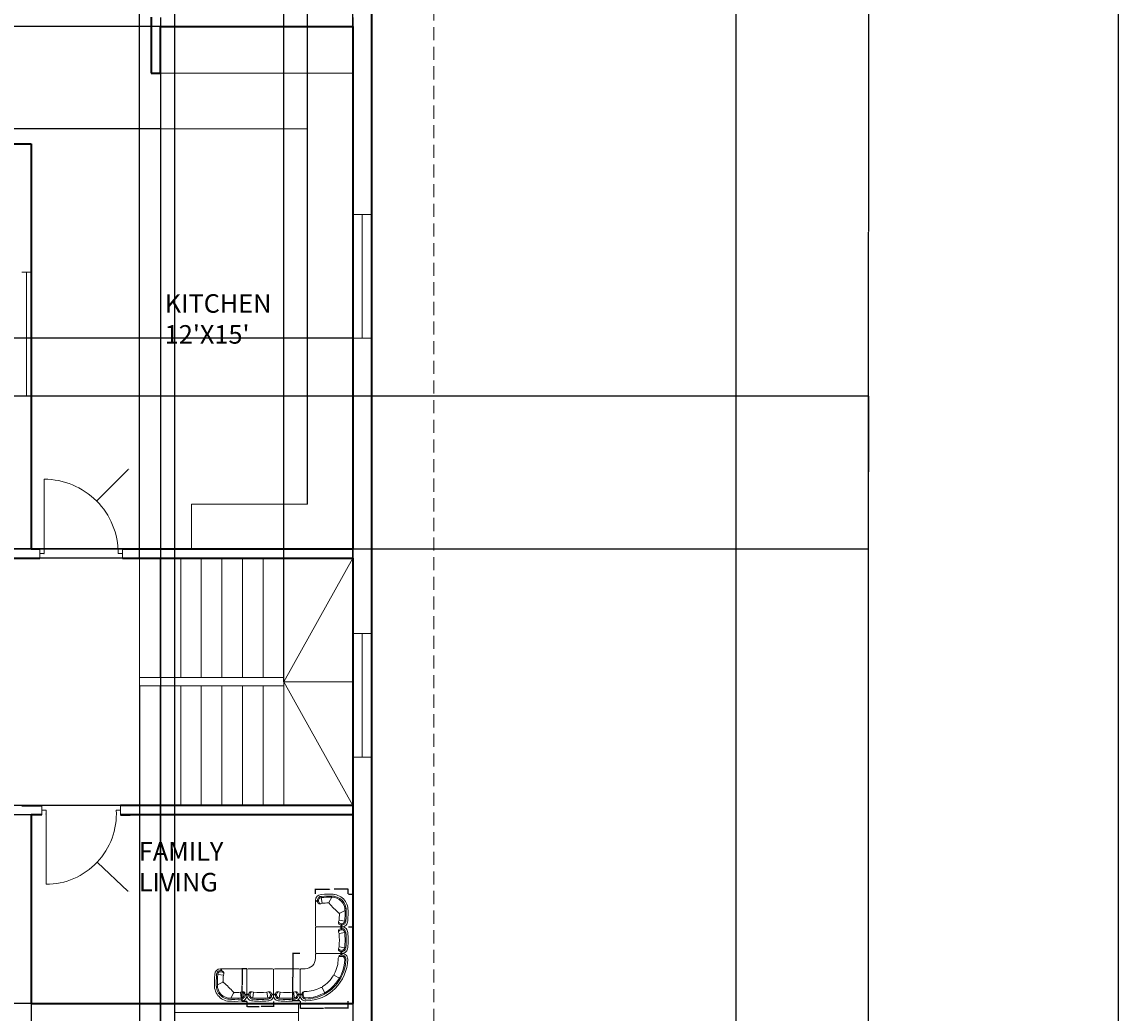
# Model space of a CAD drawing. Units: inches. Extents: x 1770 to 2988, y 1161 to 3221.
# Tile 21 of 44: x 2456 to 2988, y 1614 to 2095. Entities that reach past the tile are written whole.
import ezdxf

# ---------------------------------------------------------------- set-up
doc = ezdxf.new("R2010")
doc.units = ezdxf.units.IN
doc.linetypes.add('DASHED2', pattern=[9.525, 6.35, -3.175])
for name, color, linetype, lineweight in [('A-ANNO-DIMS', 2, 'Continuous', 18), ('A-ANNO-TTLB', 7, 'Continuous', 25), ('A-AREA-IDEN', 7, 'Continuous', 18), ('A-DOOR', 4, 'Continuous', 18), ('A-FLOR-CASE', 8, 'Continuous', 18), ('A-FLOR-STRS', 7, 'Continuous', 18), ('A-FURN', 8, 'Continuous', 13), ('A-GLAZ', 4, 'Continuous', 18), ('A-ROOF-OVHD', 7, 'DASHED2', 18), ('A-WALL', 7, 'Continuous', 35), ('C-PROP', 7, 'Continuous', 25)]:
    doc.layers.add(name, color=color, linetype=linetype, lineweight=lineweight)
doc.styles.get("Standard").update_dxf_attribs({"font": 'arial.ttf'})
doc.dimstyles.get("Standard").update_dxf_attribs({"dimtxt": 0.18, "dimasz": 0.18, "dimexe": 0.18, "dimexo": 0.0625, "dimgap": 0.09, "dimtad": 0, "dimtih": 1, "dimtoh": 1, "dimdec": 4, "dimzin": 0, "dimdsep": 46, "dimtxsty": 'Standard', "dimcen": 0.09, "dimadec": 0, "dimazin": 0, "dimtfac": 1, "dimtdec": 4, "dimtofl": 0, "dimtmove": 0, "dimatfit": 3, "dimfxl": 1, "dimtolj": 1, "dimtzin": 0, "dimarcsym": 0})

# ---------------------------------------------------------------- blocks, each defined once
blk = doc.blocks.new('A$C707258B2')
at = {"color": 0}
for p, q in [((0.404, 0.342), (1.074, 0.342)), ((0.404, 0.292), (0.454, 0.292)), ((1.104, 0.312), (1.104, 0.212)), ((0.404, 0.262), (0.454, 0.262)), ((0.6, -0.238), (0.47, -0.313)), ((1.479, -0.063), (1.379, -0.063)), ((1.509, -0.763), (1.509, -0.093)), ((0.929, -0.567), (0.854, -0.697)), ((1.429, -0.763), (1.429, -0.713)), ((1.459, -0.763), (1.459, -0.712))]:
    blk.add_line(p, q, dxfattribs=at)
for centre, radius, start, end in [((0.404, 0.192), 0.15, 90, 181.1754), ((0.404, 0.192), 0.1, 90, 181.1754), ((0.378, 0.317), 0.0362, 316.3972, 43.6028), ((0.368, 0.317), 0.0662, 337.8298, 22.1702), ((0.455, 0.256), 0.0357, 345.4262, 90.5555), ((1.074, 0.312), 0.03, 360, 90), ((1.379, 0.212), 1.125, 181.1754, 268.8246), ((1.379, 0.212), 1.075, 181.1754, 208.6357), ((0.404, 0.192), 0.07, 90, 181.1754), ((1.379, 0.212), 1.045, 181.1754, 268.8246), ((0.454, 0.212), 0.05, 360, 90), ((1.379, 0.212), 0.875, 180, 208.4082), ((1.379, 0.212), 0.275, 180, 270), ((0.587, -0.216), 0.025, 300, 28.4082), ((0.612, -0.259), 0.025, 31.5918, 120), ((1.379, 0.212), 0.875, 211.5918, 238.4082), ((1.479, -0.093), 0.03, 360, 90), ((0.457, -0.291), 0.025, 208.6357, 300), ((0.482, -0.334), 0.025, 120, 211.3643), ((1.379, 0.212), 1.075, 211.3643, 238.6357), ((0.907, -0.555), 0.025, 330, 58.4082), ((0.951, -0.58), 0.025, 61.5918, 150), ((1.379, 0.212), 0.875, 241.5918, 270), ((0.832, -0.685), 0.025, 238.6357, 330), ((0.876, -0.71), 0.025, 150, 241.3643), ((1.379, 0.212), 1.075, 241.3643, 268.8246), ((1.359, -0.763), 0.15, 268.8246, 360), ((1.359, -0.763), 0.1, 268.8246, 360), ((1.359, -0.763), 0.07, 268.8246, 360), ((1.379, -0.713), 0.05, 360, 90), ((1.425, -0.709), 0.0336, 354.6301, 109.3883), ((1.484, -0.799), 0.0662, 67.8298, 112.1702), ((1.484, -0.789), 0.0362, 46.3972, 133.6028)]:
    blk.add_arc(centre, radius, start, end, dxfattribs=at)
blk = doc.blocks.new('part 01')
at = {"color": 0}
for p, q in [((-670, 700), (0, 700)), ((30, 30), (30, 670)), ((-591, 527), (-740, 550)), ((-591, 527), (-579, 561)), ((-591, 173), (-740, 150)), ((-670, 0), (0, 0)), ((-591, 173), (-579, 139))]:
    blk.add_line(p, q, dxfattribs=at)
for centre, radius, start, end in [((-670, 550), 150, 90, 181.1754), ((-670, 550), 100, 90, 181.1754), ((-670, 550), 70, 90, 181.1754), ((-660, 518), 133, 56.0897, 95.6132), ((-696, 675), 36.2, 316.3972, 43.6028), ((-660, 518), 103, 42.0066, 95.6132), ((-706, 675), 66.2, 337.8298, 22.1702), ((-600, 607), 25, 332.9608, 56.0897), ((-625, 620), 53.2, 321.0017, 332.9608), ((-602, 570), 25, 340, 42.0066), ((0, 670), 30, 0, 90), ((1178, 350), 2008, 174.2835, 185.7165), ((1178, 350), 1958, 174.2835, 185.7165), ((1178, 350), 1928, 174.2835, 185.7165), ((1178, 350), 1778, 174.2835, 185.7165), ((-670, 150), 150, 178.8246, 270), ((-670, 150), 100, 178.8246, 270), ((-670, 150), 70, 178.8246, 270), ((-660, 182), 133, 264.3868, 303.9103), ((-660, 182), 103, 264.3868, 317.9934), ((-696, 25), 36.2, 316.3972, 43.6028), ((-706, 25), 66.2, 337.8298, 22.1702), ((-600, 93), 25, 303.9103, 27.0392), ((-602, 130), 25, 317.9934, 20), ((-625, 80), 53.2, 27.0392, 38.9983), ((0, 30), 30, 270, 0)]:
    blk.add_arc(centre, radius, start, end, dxfattribs=at)
blk = doc.blocks.new('part02')
at = {"color": 0}
for p, q in [((0, -670), (0, 0)), ((30, 30), (700, 30)), ((621, -143), (609, -109)), ((621, -143), (770, -120)), ((640, -326), (778, -399)), ((173, -591), (139, -579)), ((173, -591), (150, -740)), ((356, -610), (429, -748))]:
    blk.add_line(p, q, dxfattribs=at)
for centre, radius, start, end in [((30, 0), 30, 90, 180), ((726, 5), 56.2, 153.6122, 206.6666), ((726, 5), 36.2, 136.3972, 223.6028), ((700, -120), 150, 0, 90), ((630, -63), 25, 123.9103, 207.0392), ((655, -50), 53.2, 207.0392, 218.9983), ((632, -100), 25, 137.9934, 200), ((690, -152), 103, 84.3868, 137.9934), ((689, -151), 132, 85.4378, 123.9887), ((-1148, -320), 1778, 0.3836, 5.7165), ((700, -121), 101, 357.5006, 89.858), ((700, -120), 70, 0, 90), ((-1228, -320), 2008, 357.7349, 5.7032), ((-1148, -320), 1958, 355.8657, 5.7165), ((-1148, -320), 2008, 355.818, 5.7165), ((93, -600), 25, 62.9608, 146.0897), ((80, -625), 53.2, 51.0017, 62.9608), ((130, -602), 25, 70, 132.0066), ((2220, -2190), 2454, 130.6961, 139.3039), ((439, -409), 419, 268.2181, 1.7819), ((439, -409), 369, 268.2181, 1.7819), ((439, -409), 339, 268.2181, 1.7819), ((632, -344), 20, 62, 130.6961), ((650, -308), 20, 180.3836, 242), ((25, -696), 56.2, 63.3334, 116.3878), ((25, -696), 36.2, 46.3972, 133.6028), ((150, -670), 150, 180, 271.1754), ((182, -660), 133, 146.0897, 185.6132), ((150, -670), 100, 180, 271.1754), ((182, -660), 103, 132.0066, 185.6132), ((150, -670), 70, 180, 270), ((350, 1258), 2008, 264.2968, 272.2651), ((350, 1178), 2008, 264.2835, 274.182), ((350, 1178), 1958, 264.2835, 274.1343), ((350, 1178), 1778, 264.2835, 269.6164), ((338, -620), 20, 28, 89.6164), ((374, -602), 20, 139.3039, 208)]:
    blk.add_arc(centre, radius, start, end, dxfattribs=at)
blk = doc.blocks.new('WIN-60-EXT')
for p, q in [((0, 9), (0, 0)), ((60, 4.5), (60, 9)), ((60, 9), (60, 0)), ((0, 0), (0, 4.5)), ((0, 4.5), (60, 4.5))]:
    blk.add_line(p, q)
blk = doc.blocks.new('WIN-60-COURTYARD')
for p, q in [((0, 4.5), (0, 0)), ((0, 0), (0, 2.25)), ((0, 2.25), (60, 2.25)), ((60, 2.25), (60, 4.5)), ((60, 4.5), (60, 0))]:
    blk.add_line(p, q)
blk = doc.blocks.new('*D44')
at = {"layer": 'A-ANNO-DIMS', "color": 0, "lineweight": -2, "transparency": 16777216}
for p, q in [((2565.27, 1635.99), (2562.77, 1635.99)), ((2562.95, 1635.81), (2562.95, 1628.23)), ((2562.95, 1620.29), (2562.95, 1627.87)), ((2565.27, 1620.11), (2562.77, 1620.11))]:
    blk.add_line(p, q, dxfattribs=at)
at = {"layer": 'A-ANNO-DIMS', "color": 0, "transparency": 16777216}
for points in [[(2562.92, 1635.81), (2562.98, 1635.81), (2562.95, 1635.99)], [(2562.92, 1620.29), (2562.98, 1620.29), (2562.95, 1620.11)]]:
    blk.add_solid(points, dxfattribs=at)
at = {"layer": 'Defpoints', "color": 0, "transparency": 16777216}
for p in [(2562.95, 1635.99), (2565.33, 1635.99), (2565.33, 1620.11)]:
    blk.add_point(p, dxfattribs=at)
at = {"layer": 'A-ANNO-DIMS', "color": 0, "transparency": 16777216, "insert": (2562.95, 1628.05), "char_height": 0.18, "attachment_point": 5}
blk.add_mtext('\\A1;SEAT 16 TYP.', dxfattribs=at)
blk = doc.blocks.new('*D45')
at = {"layer": 'A-ANNO-DIMS', "color": 0, "lineweight": -2, "transparency": 16777216}
for p, q in [((2565.33, 1620.05), (2565.33, 1617.55)), ((2565.51, 1617.73), (2571.25, 1617.73)), ((2578.04, 1617.73), (2572.29, 1617.73)), ((2578.22, 1620.05), (2578.22, 1617.55))]:
    blk.add_line(p, q, dxfattribs=at)
at = {"layer": 'A-ANNO-DIMS', "color": 0, "transparency": 16777216}
for points in [[(2565.51, 1617.76), (2565.51, 1617.7), (2565.33, 1617.73)], [(2578.04, 1617.76), (2578.04, 1617.7), (2578.22, 1617.73)]]:
    blk.add_solid(points, dxfattribs=at)
at = {"layer": 'Defpoints', "color": 0, "transparency": 16777216}
for p in [(2565.33, 1620.11), (2565.33, 1617.73), (2578.22, 1620.11)]:
    blk.add_point(p, dxfattribs=at)
at = {"layer": 'A-ANNO-DIMS', "color": 0, "transparency": 16777216, "insert": (2571.77, 1617.73), "char_height": 0.18, "attachment_point": 5}
blk.add_mtext('\\A1;13 TYP.', dxfattribs=at)
blk = doc.blocks.new('*D46')
at = {"layer": 'A-ANNO-DIMS', "color": 0, "lineweight": -2, "transparency": 16777216}
for p, q in [((2598.55, 1672.27), (2598.55, 1674.77)), ((2598.73, 1674.59), (2605.3, 1674.59)), ((2614.25, 1674.59), (2607.68, 1674.59)), ((2614.43, 1672.27), (2614.43, 1674.77))]:
    blk.add_line(p, q, dxfattribs=at)
at = {"layer": 'A-ANNO-DIMS', "color": 0, "transparency": 16777216}
for points in [[(2598.73, 1674.62), (2598.73, 1674.56), (2598.55, 1674.59)], [(2614.25, 1674.62), (2614.25, 1674.56), (2614.43, 1674.59)]]:
    blk.add_solid(points, dxfattribs=at)
at = {"layer": 'Defpoints', "color": 0, "transparency": 16777216}
for p in [(2598.55, 1674.59), (2598.55, 1672.2), (2614.43, 1672.2)]:
    blk.add_point(p, dxfattribs=at)
at = {"layer": 'A-ANNO-DIMS', "color": 0, "transparency": 16777216, "insert": (2606.49, 1674.59), "char_height": 0.18, "attachment_point": 5}
blk.add_mtext('\\A1;END SEAT 16 TYP.', dxfattribs=at)
blk = doc.blocks.new('*D47')
at = {"layer": 'A-ANNO-DIMS', "color": 0, "lineweight": -2, "transparency": 16777216}
for p, q in [((2614.49, 1672.2), (2616.99, 1672.2)), ((2616.81, 1672.02), (2616.81, 1664.45)), ((2616.81, 1656.51), (2616.81, 1664.08)), ((2614.49, 1656.33), (2616.99, 1656.33))]:
    blk.add_line(p, q, dxfattribs=at)
at = {"layer": 'A-ANNO-DIMS', "color": 0, "transparency": 16777216}
for points in [[(2616.78, 1672.02), (2616.84, 1672.02), (2616.81, 1672.2)], [(2616.78, 1656.51), (2616.84, 1656.51), (2616.81, 1656.33)]]:
    blk.add_solid(points, dxfattribs=at)
at = {"layer": 'Defpoints', "color": 0, "transparency": 16777216}
for p in [(2614.43, 1672.2), (2616.81, 1672.2), (2614.43, 1656.33)]:
    blk.add_point(p, dxfattribs=at)
at = {"layer": 'A-ANNO-DIMS', "color": 0, "transparency": 16777216, "insert": (2616.81, 1664.27), "char_height": 0.18, "attachment_point": 5}
blk.add_mtext('\\A1;16 TYP.', dxfattribs=at)
blk = doc.blocks.new('*D48')
at = {"layer": 'A-ANNO-DIMS', "color": 0, "lineweight": -2, "transparency": 16777216}
for p, q in [((2591.03, 1643.44), (2587.45, 1643.44)), ((2587.63, 1643.26), (2587.63, 1632.08)), ((2587.63, 1620.52), (2587.63, 1631.71)), ((2591.03, 1620.34), (2587.45, 1620.34))]:
    blk.add_line(p, q, dxfattribs=at)
at = {"layer": 'A-ANNO-DIMS', "color": 0, "transparency": 16777216}
for points in [[(2587.6, 1643.26), (2587.66, 1643.26), (2587.63, 1643.44)], [(2587.6, 1620.52), (2587.66, 1620.52), (2587.63, 1620.34)]]:
    blk.add_solid(points, dxfattribs=at)
at = {"layer": 'Defpoints', "color": 0, "transparency": 16777216}
for p in [(2587.63, 1643.44), (2591.1, 1643.44), (2591.1, 1620.34)]:
    blk.add_point(p, dxfattribs=at)
at = {"layer": 'A-ANNO-DIMS', "color": 0, "transparency": 16777216, "insert": (2587.63, 1631.89), "char_height": 0.18, "attachment_point": 5}
blk.add_mtext('\\A1;CORNER SEAT 23', dxfattribs=at)
blk = doc.blocks.new('*D49')
at = {"layer": 'A-ANNO-DIMS', "color": 0, "lineweight": -2, "transparency": 16777216}
for p, q in [((2591.1, 1620.28), (2591.1, 1616.69)), ((2591.28, 1616.87), (2602.43, 1616.87)), ((2614.02, 1616.87), (2602.87, 1616.87)), ((2614.2, 1620.28), (2614.2, 1616.69))]:
    blk.add_line(p, q, dxfattribs=at)
at = {"layer": 'A-ANNO-DIMS', "color": 0, "transparency": 16777216}
for points in [[(2591.28, 1616.9), (2591.28, 1616.84), (2591.1, 1616.87)], [(2614.02, 1616.9), (2614.02, 1616.84), (2614.2, 1616.87)]]:
    blk.add_solid(points, dxfattribs=at)
at = {"layer": 'Defpoints', "color": 0, "transparency": 16777216}
for p in [(2591.1, 1620.34), (2591.1, 1616.87), (2614.2, 1620.34)]:
    blk.add_point(p, dxfattribs=at)
at = {"layer": 'A-ANNO-DIMS', "color": 0, "transparency": 16777216, "insert": (2602.65, 1616.87), "char_height": 0.18, "attachment_point": 5}
blk.add_mtext('\\A1;23', dxfattribs=at)
blk = doc.blocks.new('*D61')
at = {"layer": 'A-ANNO-DIMS', "color": 0, "lineweight": -2, "transparency": 16777216}
for p, q in [((2625.76, 2376.7), (2866.87, 2376.7)), ((2866.69, 2376.52), (2866.69, 1993.63)), ((2866.69, 1610.38), (2866.69, 1993.27)), ((2625.76, 1610.2), (2866.87, 1610.2))]:
    blk.add_line(p, q, dxfattribs=at)
at = {"layer": 'A-ANNO-DIMS', "color": 0, "transparency": 16777216}
for points in [[(2866.66, 2376.52), (2866.72, 2376.52), (2866.69, 2376.7)], [(2866.66, 1610.38), (2866.72, 1610.38), (2866.69, 1610.2)]]:
    blk.add_solid(points, dxfattribs=at)
at = {"layer": 'Defpoints', "color": 0, "transparency": 16777216}
for p in [(2625.7, 2376.7), (2866.69, 2376.7), (2625.7, 1610.2)]:
    blk.add_point(p, dxfattribs=at)
at = {"layer": 'A-ANNO-DIMS', "color": 0, "transparency": 16777216, "insert": (2866.69, 1993.45), "char_height": 0.18, "attachment_point": 5}
blk.add_mtext('\\A1;766.5', dxfattribs=at)
blk = doc.blocks.new('*D74')
at = {"layer": 'A-ANNO-DIMS', "color": 0, "lineweight": -2, "transparency": 16777216}
for p, q in [((2523.42, 2097.48), (2523.42, 1165.57)), ((2616.7, 2097.48), (2616.7, 1165.57)), ((2523.6, 1165.75), (2569.66, 1165.75)), ((2616.52, 1165.75), (2570.45, 1165.75))]:
    blk.add_line(p, q, dxfattribs=at)
at = {"layer": 'A-ANNO-DIMS', "color": 0, "transparency": 16777216}
for points in [[(2523.6, 1165.78), (2523.6, 1165.72), (2523.42, 1165.75)], [(2616.52, 1165.78), (2616.52, 1165.72), (2616.7, 1165.75)]]:
    blk.add_solid(points, dxfattribs=at)
at = {"layer": 'Defpoints', "color": 0, "transparency": 16777216}
for p in [(2523.42, 2097.54), (2616.7, 2097.54), (2616.7, 1165.75)]:
    blk.add_point(p, dxfattribs=at)
at = {"layer": 'A-ANNO-DIMS', "color": 0, "transparency": 16777216, "insert": (2570.06, 1165.75), "char_height": 0.18, "attachment_point": 5}
blk.add_mtext('\\A1;93.28', dxfattribs=at)
blk = doc.blocks.new('*D76')
at = {"layer": 'A-ANNO-DIMS', "color": 0, "lineweight": -2, "transparency": 16777216}
for p, q in [((2460.63, 1710.7), (1907.1, 1710.7)), ((1907.28, 1710.52), (1907.28, 1665.13)), ((1907.28, 1619.38), (1907.28, 1664.77)), ((2460.63, 1619.2), (1907.1, 1619.2))]:
    blk.add_line(p, q, dxfattribs=at)
at = {"layer": 'A-ANNO-DIMS', "color": 0, "transparency": 16777216}
for points in [[(1907.25, 1710.52), (1907.31, 1710.52), (1907.28, 1710.7)], [(1907.25, 1619.38), (1907.31, 1619.38), (1907.28, 1619.2)]]:
    blk.add_solid(points, dxfattribs=at)
at = {"layer": 'Defpoints', "color": 0, "transparency": 16777216}
for p in [(1907.28, 1710.7), (2460.7, 1710.7), (2460.7, 1619.2)]:
    blk.add_point(p, dxfattribs=at)
at = {"layer": 'A-ANNO-DIMS', "color": 0, "transparency": 16777216, "insert": (1907.28, 1664.95), "char_height": 0.18, "attachment_point": 5}
blk.add_mtext('\\A1;91.5', dxfattribs=at)
blk = doc.blocks.new('*D77')
at = {"layer": 'A-ANNO-DIMS', "color": 0, "lineweight": -2, "transparency": 16777216}
for p, q in [((2460.7, 1710.64), (2460.7, 1165.57)), ((2616.7, 1710.64), (2616.7, 1165.57)), ((2460.88, 1165.75), (2538.42, 1165.75)), ((2616.52, 1165.75), (2538.98, 1165.75))]:
    blk.add_line(p, q, dxfattribs=at)
at = {"layer": 'A-ANNO-DIMS', "color": 0, "transparency": 16777216}
for points in [[(2460.88, 1165.78), (2460.88, 1165.72), (2460.7, 1165.75)], [(2616.52, 1165.78), (2616.52, 1165.72), (2616.7, 1165.75)]]:
    blk.add_solid(points, dxfattribs=at)
at = {"layer": 'Defpoints', "color": 0, "transparency": 16777216}
for p in [(2460.7, 1710.7), (2616.7, 1710.7), (2616.7, 1165.75)]:
    blk.add_point(p, dxfattribs=at)
at = {"layer": 'A-ANNO-DIMS', "color": 0, "transparency": 16777216, "insert": (2538.7, 1165.75), "char_height": 0.18, "attachment_point": 5}
blk.add_mtext('\\A1;156', dxfattribs=at)
blk = doc.blocks.new('*D82')
at = {"layer": 'A-ANNO-DIMS', "color": 0, "lineweight": -2, "transparency": 16777216}
for p, q in [((2443.39, 1610.26), (2443.39, 2570.7)), ((2443.57, 2570.52), (2486.45, 2570.52)), ((2530.12, 2570.52), (2487.24, 2570.52)), ((2530.3, 1610.26), (2530.3, 2570.7))]:
    blk.add_line(p, q, dxfattribs=at)
at = {"layer": 'A-ANNO-DIMS', "color": 0, "transparency": 16777216}
for points in [[(2443.57, 2570.55), (2443.57, 2570.49), (2443.39, 2570.52)], [(2530.12, 2570.55), (2530.12, 2570.49), (2530.3, 2570.52)]]:
    blk.add_solid(points, dxfattribs=at)
at = {"layer": 'Defpoints', "color": 0, "transparency": 16777216}
for p in [(2530.3, 2570.52), (2443.39, 1610.2), (2530.3, 1610.2)]:
    blk.add_point(p, dxfattribs=at)
at = {"layer": 'A-ANNO-DIMS', "color": 0, "transparency": 16777216, "insert": (2486.85, 2570.52), "char_height": 0.18, "attachment_point": 5}
blk.add_mtext('\\A1;86.92', dxfattribs=at)
blk = doc.blocks.new('*D83')
at = {"layer": 'A-ANNO-DIMS', "color": 0, "lineweight": -2, "transparency": 16777216}
for p, q in [((2513.13, 1835.2), (1907.1, 1835.2)), ((1907.28, 1835.02), (1907.28, 1775.38)), ((1907.28, 1715.38), (1907.28, 1775.02)), ((2513.13, 1715.2), (1907.1, 1715.2))]:
    blk.add_line(p, q, dxfattribs=at)
at = {"layer": 'A-ANNO-DIMS', "color": 0, "transparency": 16777216}
for points in [[(1907.25, 1835.02), (1907.31, 1835.02), (1907.28, 1835.2)], [(1907.25, 1715.38), (1907.31, 1715.38), (1907.28, 1715.2)]]:
    blk.add_solid(points, dxfattribs=at)
at = {"layer": 'Defpoints', "color": 0, "transparency": 16777216}
for p in [(1907.28, 1835.2), (2513.2, 1835.2), (2513.2, 1715.2)]:
    blk.add_point(p, dxfattribs=at)
at = {"layer": 'A-ANNO-DIMS', "color": 0, "transparency": 16777216, "insert": (1907.28, 1775.2), "char_height": 0.18, "attachment_point": 5}
blk.add_mtext('\\A1;120', dxfattribs=at)
blk = doc.blocks.new('*D84')
at = {"layer": 'A-ANNO-DIMS', "color": 0, "lineweight": -2, "transparency": 16777216}
for p, q in [((2513.2, 1835.26), (2513.2, 2570.7)), ((2513.38, 2570.52), (2564.56, 2570.52)), ((2616.52, 2570.52), (2565.33, 2570.52)), ((2616.7, 1835.26), (2616.7, 2570.7))]:
    blk.add_line(p, q, dxfattribs=at)
at = {"layer": 'A-ANNO-DIMS', "color": 0, "transparency": 16777216}
for points in [[(2513.38, 2570.55), (2513.38, 2570.49), (2513.2, 2570.52)], [(2616.52, 2570.55), (2616.52, 2570.49), (2616.7, 2570.52)]]:
    blk.add_solid(points, dxfattribs=at)
at = {"layer": 'Defpoints', "color": 0, "transparency": 16777216}
for p in [(2616.7, 2570.52), (2513.2, 1835.2), (2616.7, 1835.2)]:
    blk.add_point(p, dxfattribs=at)
at = {"layer": 'A-ANNO-DIMS', "color": 0, "transparency": 16777216, "insert": (2564.95, 2570.52), "char_height": 0.18, "attachment_point": 5}
blk.add_mtext('\\A1;103.5', dxfattribs=at)
blk = doc.blocks.new('*D85')
at = {"layer": 'A-ANNO-DIMS', "color": 0, "lineweight": -2, "transparency": 16777216}
for p, q in [((2513.2, 1773.14), (2513.2, 1165.57)), ((2523.2, 1773.14), (2523.2, 1165.57)), ((2513.38, 1165.75), (2517.99, 1165.75)), ((2523.02, 1165.75), (2518.41, 1165.75))]:
    blk.add_line(p, q, dxfattribs=at)
at = {"layer": 'A-ANNO-DIMS', "color": 0, "transparency": 16777216}
for points in [[(2513.38, 1165.78), (2513.38, 1165.72), (2513.2, 1165.75)], [(2523.02, 1165.78), (2523.02, 1165.72), (2523.2, 1165.75)]]:
    blk.add_solid(points, dxfattribs=at)
at = {"layer": 'Defpoints', "color": 0, "transparency": 16777216}
for p in [(2513.2, 1773.2), (2523.2, 1773.2), (2523.2, 1165.75)]:
    blk.add_point(p, dxfattribs=at)
at = {"layer": 'A-ANNO-DIMS', "color": 0, "transparency": 16777216, "insert": (2518.2, 1165.75), "char_height": 0.18, "attachment_point": 5}
blk.add_mtext('\\A1;10', dxfattribs=at)
blk = doc.blocks.new('*D86')
at = {"layer": 'A-ANNO-DIMS', "color": 0, "lineweight": -2, "transparency": 16777216}
for p, q in [((2583.2, 1775.21), (2583.2, 2570.7)), ((2583.38, 2570.52), (2599.62, 2570.52)), ((2616.52, 2570.52), (2600.27, 2570.52)), ((2616.7, 1775.26), (2616.7, 2570.7))]:
    blk.add_line(p, q, dxfattribs=at)
at = {"layer": 'A-ANNO-DIMS', "color": 0, "transparency": 16777216}
for points in [[(2583.38, 2570.55), (2583.38, 2570.49), (2583.2, 2570.52)], [(2616.52, 2570.55), (2616.52, 2570.49), (2616.7, 2570.52)]]:
    blk.add_solid(points, dxfattribs=at)
at = {"layer": 'Defpoints', "color": 0, "transparency": 16777216}
for p in [(2616.7, 2570.52), (2583.2, 1775.15), (2616.7, 1775.2)]:
    blk.add_point(p, dxfattribs=at)
at = {"layer": 'A-ANNO-DIMS', "color": 0, "transparency": 16777216, "insert": (2599.95, 2570.52), "char_height": 0.18, "attachment_point": 5}
blk.add_mtext('\\A1;33.5', dxfattribs=at)
blk = doc.blocks.new('*D87')
at = {"layer": 'A-ANNO-DIMS', "color": 0, "lineweight": -2, "transparency": 16777216}
for p, q in [((2594.75, 1861.4), (2594.75, 2570.7)), ((2594.93, 2570.52), (2605.33, 2570.52)), ((2616.52, 2570.52), (2606.12, 2570.52)), ((2616.7, 1839.76), (2616.7, 2570.7))]:
    blk.add_line(p, q, dxfattribs=at)
at = {"layer": 'A-ANNO-DIMS', "color": 0, "transparency": 16777216}
for points in [[(2594.93, 2570.55), (2594.93, 2570.49), (2594.75, 2570.52)], [(2616.52, 2570.55), (2616.52, 2570.49), (2616.7, 2570.52)]]:
    blk.add_solid(points, dxfattribs=at)
at = {"layer": 'Defpoints', "color": 0, "transparency": 16777216}
for p in [(2616.7, 2570.52), (2594.75, 1861.34), (2616.7, 1839.7)]:
    blk.add_point(p, dxfattribs=at)
at = {"layer": 'A-ANNO-DIMS', "color": 0, "transparency": 16777216, "insert": (2605.72, 2570.52), "char_height": 0.18, "attachment_point": 5}
blk.add_mtext('\\A1;21.95', dxfattribs=at)
blk = doc.blocks.new('*D88')
at = {"layer": 'A-ANNO-DIMS', "color": 0, "lineweight": -2, "transparency": 16777216}
for p, q in [((2523.36, 2093.04), (1907.1, 2093.04)), ((1907.28, 2092.86), (1907.28, 2068.4)), ((1907.28, 2043.57), (1907.28, 2068.04)), ((2523.36, 2043.39), (1907.1, 2043.39))]:
    blk.add_line(p, q, dxfattribs=at)
at = {"layer": 'A-ANNO-DIMS', "color": 0, "transparency": 16777216}
for points in [[(1907.25, 2092.86), (1907.31, 2092.86), (1907.28, 2093.04)], [(1907.25, 2043.57), (1907.31, 2043.57), (1907.28, 2043.39)]]:
    blk.add_solid(points, dxfattribs=at)
at = {"layer": 'Defpoints', "color": 0, "transparency": 16777216}
for p in [(1907.28, 2093.04), (2523.42, 2093.04), (2523.42, 2043.39)]:
    blk.add_point(p, dxfattribs=at)
at = {"layer": 'A-ANNO-DIMS', "color": 0, "transparency": 16777216, "insert": (1907.28, 2068.22), "char_height": 0.18, "attachment_point": 5}
blk.add_mtext('\\A1;49.65', dxfattribs=at)
blk = doc.blocks.new('*D90')
at = {"layer": 'A-ANNO-DIMS', "color": 0, "lineweight": -2, "transparency": 16777216}
for p, q in [((2616.63, 1941.8), (1907.1, 1941.8)), ((1907.28, 1941.62), (1907.28, 1890.93)), ((1907.28, 1839.88), (1907.28, 1890.57)), ((2616.63, 1839.7), (1907.1, 1839.7))]:
    blk.add_line(p, q, dxfattribs=at)
at = {"layer": 'A-ANNO-DIMS', "color": 0, "transparency": 16777216}
for points in [[(1907.25, 1941.62), (1907.31, 1941.62), (1907.28, 1941.8)], [(1907.25, 1839.88), (1907.31, 1839.88), (1907.28, 1839.7)]]:
    blk.add_solid(points, dxfattribs=at)
at = {"layer": 'Defpoints', "color": 0, "transparency": 16777216}
for p in [(1907.28, 1941.8), (2616.7, 1941.8), (2616.7, 1839.7)]:
    blk.add_point(p, dxfattribs=at)
at = {"layer": 'A-ANNO-DIMS', "color": 0, "transparency": 16777216, "insert": (1907.28, 1890.75), "char_height": 0.18, "attachment_point": 5}
blk.add_mtext('\\A1;102.1', dxfattribs=at)
blk = doc.blocks.new('*D92')
at = {"layer": 'A-ANNO-DIMS', "color": 0, "lineweight": -2, "transparency": 16777216}
for p, q in [((2333.26, 1913.9), (2866.87, 1913.9)), ((2866.69, 1913.72), (2866.69, 1876.98)), ((2866.69, 1839.88), (2866.69, 1876.62)), ((2333.26, 1839.7), (2866.87, 1839.7))]:
    blk.add_line(p, q, dxfattribs=at)
at = {"layer": 'A-ANNO-DIMS', "color": 0, "transparency": 16777216}
for points in [[(2866.66, 1913.72), (2866.72, 1913.72), (2866.69, 1913.9)], [(2866.66, 1839.88), (2866.72, 1839.88), (2866.69, 1839.7)]]:
    blk.add_solid(points, dxfattribs=at)
at = {"layer": 'Defpoints', "color": 0, "transparency": 16777216}
for p in [(2333.2, 1913.9), (2866.69, 1913.9), (2333.2, 1839.7)]:
    blk.add_point(p, dxfattribs=at)
at = {"layer": 'A-ANNO-DIMS', "color": 0, "transparency": 16777216, "insert": (2866.69, 1876.8), "char_height": 0.18, "attachment_point": 5}
blk.add_mtext('\\A1;74.2', dxfattribs=at)
blk = doc.blocks.new('*D115')
at = {"layer": 'A-ANNO-DIMS', "color": 0, "lineweight": -2, "transparency": 16777216}
for p, q in [((2507.64, 1878.17), (2492.5, 1863.03)), ((2507.82, 1878.17), (2507.64, 1878.17)), ((2466.83, 1837.47), (2467.01, 1837.47)), ((2466.92, 1837.38), (2466.92, 1837.56))]:
    blk.add_line(p, q, dxfattribs=at)
at = {"layer": 'A-ANNO-DIMS', "color": 0, "transparency": 16777216}
blk.add_solid([(2492.48, 1863.06), (2492.52, 1863.01), (2492.37, 1862.91)], dxfattribs=at)
at = {"layer": 'Defpoints', "color": 0, "transparency": 16777216}
for p in [(2492.37, 1862.91), (2466.92, 1837.47)]:
    blk.add_point(p, dxfattribs=at)
at = {"layer": 'A-ANNO-DIMS', "color": 0, "transparency": 16777216, "insert": (2508.37, 1878.17), "char_height": 0.18, "attachment_point": 5}
blk.add_mtext('\\A1;R35.985', dxfattribs=at)
blk = doc.blocks.new('*D116')
at = {"layer": 'A-ANNO-DIMS', "color": 0, "lineweight": -2, "transparency": 16777216}
for p, q in [((2467.8, 1711.04), (2467.98, 1711.04)), ((2467.89, 1710.95), (2467.89, 1711.13)), ((2507.53, 1673.57), (2492.8, 1687.5)), ((2507.71, 1673.57), (2507.53, 1673.57))]:
    blk.add_line(p, q, dxfattribs=at)
at = {"layer": 'A-ANNO-DIMS', "color": 0, "transparency": 16777216}
blk.add_solid([(2492.82, 1687.52), (2492.78, 1687.48), (2492.67, 1687.62)], dxfattribs=at)
at = {"layer": 'Defpoints', "color": 0, "transparency": 16777216}
for p in [(2467.89, 1711.04), (2492.67, 1687.62)]:
    blk.add_point(p, dxfattribs=at)
at = {"layer": 'A-ANNO-DIMS', "color": 0, "transparency": 16777216, "insert": (2508.19, 1673.57), "char_height": 0.18, "attachment_point": 5}
blk.add_mtext('\\A1;R34.09', dxfattribs=at)

msp = doc.modelspace()

# ---------------------------------------------------------------- linework, layer by layer
at = {"layer": 'A-ANNO-TTLB'}
msp.add_lwpolyline([(1769.9155, 3221.2788), (2987.7567, 3221.2788), (2987.7567, 1161.1516), (1769.9155, 1161.1516)], close=True, dxfattribs=at)
at = {"layer": 'A-DOOR'}
for p, q in [((2466.9215, 1837.4521), (2466.9215, 1873.4521)), ((2464.9215, 1839.7021), (2464.9215, 1835.2021)), ((2504.9069, 1839.7021), (2504.9069, 1835.2021)), ((2464.9215, 1837.4521), (2466.9215, 1837.4521)), ((2504.9069, 1837.4521), (2502.9069, 1837.4521)), ((2465.8944, 1715.2021), (2465.8944, 1710.7021)), ((2465.8944, 1712.9521), (2467.8944, 1712.9521)), ((2467.8944, 1712.9521), (2467.8944, 1676.9521)), ((2503.9305, 1712.9521), (2501.9305, 1712.9521)), ((2503.9305, 1715.2021), (2503.9305, 1710.7021))]:
    msp.add_line(p, q, dxfattribs=at)
for centre, radius, start, end in [((2466.9215, 1837.4667), 35.9854, 359.976796, 90), ((2467.8944, 1711.0418), 34.0896, 270, 3.212509)]:
    msp.add_arc(centre, radius, start, end, dxfattribs=at)
at = {"layer": 'A-FLOR-CASE'}
for p, q in [((2523.4179, 2070.4236), (2616.696, 2070.4236)), ((2523.4179, 2043.391), (2523.4179, 2070.4236)), ((2594.7479, 2043.391), (2523.4179, 2043.391)), ((2594.7479, 1861.3395), (2594.7479, 2043.391)), ((2538.3919, 1839.7021), (2538.3919, 1861.3395)), ((2538.3919, 1861.3395), (2594.7479, 1861.3395))]:
    msp.add_line(p, q, dxfattribs=at)
at = {"layer": 'A-FLOR-STRS'}
for p, q in [((2513.196, 1835.2021), (2513.196, 1773.2021)), ((2523.196, 1835.2021), (2523.196, 1777.2021)), ((2533.196, 1835.2021), (2533.196, 1777.2021)), ((2543.196, 1835.2021), (2543.196, 1777.2021)), ((2553.196, 1835.2021), (2553.196, 1777.2021)), ((2563.196, 1835.2021), (2563.196, 1777.2021)), ((2573.196, 1835.2021), (2573.196, 1777.2021)), ((2583.196, 1835.2021), (2583.196, 1773.2021)), ((2583.196, 1775.149), (2616.696, 1835.2021)), ((2616.696, 1835.2021), (2616.696, 1715.2021)), ((2583.196, 1777.2021), (2513.196, 1777.2021)), ((2513.196, 1777.2021), (2513.196, 1775.2021)), ((2616.696, 1775.2021), (2616.696, 1777.2021)), ((2513.196, 1775.2021), (2513.196, 1773.2021)), ((2513.196, 1773.2021), (2583.196, 1773.2021)), ((2513.196, 1773.2021), (2513.196, 1715.2021)), ((2523.196, 1773.2021), (2523.196, 1715.2021)), ((2533.196, 1773.2021), (2533.196, 1715.2021)), ((2543.196, 1773.2021), (2543.196, 1715.2021)), ((2553.196, 1773.2021), (2553.196, 1715.2021)), ((2563.196, 1773.2021), (2563.196, 1715.2021)), ((2573.196, 1773.2021), (2573.196, 1715.2021)), ((2583.196, 1775.149), (2616.696, 1775.149)), ((2583.196, 1775.149), (2616.696, 1715.2021)), ((2583.196, 1773.2021), (2583.196, 1715.2021))]:
    msp.add_line(p, q, dxfattribs=at)
at = {"layer": 'A-ROOF-OVHD'}
msp.add_line((2656.0216, 1610.2021), (2656.0216, 2405.7876), dxfattribs=at)
at = {"layer": 'A-WALL'}
for p, q in [((2625.696, 2376.7021), (2625.696, 1610.2021)), ((2518.9179, 2097.5443), (2518.9179, 2070.4236)), ((2523.4179, 2093.0443), (2616.696, 2093.0443)), ((2523.4179, 2070.4236), (2523.4179, 2093.0443)), ((2616.696, 2093.0443), (2616.696, 1839.7021)), ((2616.696, 2093.0443), (2616.696, 2085.13)), ((2518.9179, 2070.4236), (2523.4179, 2070.4236)), ((2328.696, 2036.2021), (2460.696, 2036.2021)), ((2460.696, 2036.2021), (2460.696, 1839.7021)), ((2460.696, 1839.7021), (2464.9215, 1839.7021)), ((2504.9069, 1839.7021), (2616.696, 1839.7021)), ((2328.696, 1835.2021), (2464.9215, 1835.2021)), ((2460.696, 1835.2021), (2464.9215, 1835.2021)), ((2504.9069, 1835.2021), (2616.696, 1835.2021)), ((2504.9069, 1835.2021), (2508.696, 1835.2021)), ((2616.696, 1835.2021), (2616.696, 1619.2021)), ((2456.196, 1715.2021), (2460.696, 1715.2021)), ((2460.696, 1715.2021), (2465.8944, 1715.2021)), ((2508.696, 1715.2021), (2503.9305, 1715.2021)), ((2616.696, 1715.2021), (2508.696, 1715.2021)), ((2460.696, 1710.7021), (2460.696, 1619.2021)), ((2465.8944, 1710.7021), (2460.696, 1710.7021)), ((2616.696, 1710.7021), (2503.9305, 1710.7021)), ((2503.9305, 1710.7021), (2508.696, 1710.7021)), ((2460.696, 1619.2021), (2616.696, 1619.2021))]:
    msp.add_line(p, q, dxfattribs=at)
at = {"layer": 'C-PROP'}
msp.add_lwpolyline([(1971.5344, 2506.2747), (2802.4374, 2506.2747), (2802.4374, 1323.5288), (1971.5344, 1323.5288)], close=True, dxfattribs=at)

# ---------------------------------------------------------------- block references
at = {"layer": 'A-FURN', "ltscale": 0.03}
for name, p, xscale, yscale, zscale, rotation in [('part02', (2599.1017, 1656.3262), 0.0184021866095898, 0.0184021866095898, 0.0184021866095898, 90), ('part 01', (2599.1017, 1656.3262), 0.0184021866095898, 0.0184021866095898, 0.0184021866095898, 180), ('A$C707258B2', (2618.8646, 1637.1508), -18.40218660958979, 18.40218660958979, 18.40218660958979, 359.9999999999968), ('part02', (2565.3337, 1635.4397), -0.0184021866095898, 0.0184021866095898, 0.0184021866095898, 359.9999999999968), ('part 01', (2578.2152, 1635.4397), 0.0184021866095898, 0.0184021866095898, 0.0184021866095898, 90), ('part 01', (2591.0967, 1635.4397), 0.0184021866095898, 0.0184021866095898, 0.0184021866095898, 90)]:
    msp.add_blockref(name, p, dxfattribs=dict(at, xscale=xscale, yscale=yscale, zscale=zscale, rotation=rotation))
at = {"layer": 'A-GLAZ', "extrusion": (0, 0, -1), "zscale": -1, "rotation": 90}
for name, p in [('WIN-60-EXT', (-2616.6958, 1941.8006)), ('WIN-60-COURTYARD', (-2456.1958, 1913.8992))]:
    msp.add_blockref(name, p, dxfattribs=at)
at = {"layer": 'A-GLAZ', "rotation": 90}
msp.add_blockref('WIN-60-EXT', (2625.6961, 1738.6495), dxfattribs=at)
at = {"layer": 'A-GLAZ'}
msp.add_blockref('WIN-60-EXT', (2530.304, 1610.202), dxfattribs=at)

# ---------------------------------------------------------------- texts
at = {"layer": 'A-AREA-IDEN', "char_height": 9, "attachment_point": 1}
for s, width, insert in [("KITCHEN\\P12'X15'", 104.831201, (2525.4551, 1963.2061)), ('FAMILY LIVING', 80.373863, (2512.8935, 1697.4705))]:
    msp.add_mtext_dynamic_manual_height_columns(s, width=width, gutter_width=12.5, heights=[0], dxfattribs=dict(at, insert=insert))

# ---------------------------------------------------------------- dimensions: what is measured, and where the dimension line sits
at = {"layer": 'A-ANNO-DIMS'}
for base, p1, p2, override, picture, middle in [((2530.3038, 2570.5247), (2443.3863, 1610.2021), (2530.3038, 1610.2021), {"dimdec": 2, "dimlfac": 1, "dimrnd": 0, "dimzin": 0, "dimdsep": 46, "dimlunit": 2}, '*D82', (2486.8451, 2570.5247)), ((2616.696, 2570.5247), (2513.196, 1835.2021), (2616.696, 1835.2021), {"dimdec": 1, "dimlfac": 1, "dimrnd": 0, "dimzin": 0, "dimdsep": 46, "dimlunit": 2}, '*D84', (2564.946, 2570.5247)), ((2616.696, 2570.5247), (2583.196, 1775.149), (2616.696, 1775.2021), {"dimdec": 1, "dimlfac": 1, "dimrnd": 0, "dimzin": 0, "dimdsep": 46, "dimlunit": 2}, '*D86', (2599.946, 2570.5247)), ((2616.696, 2570.5247), (2594.7479, 1861.3395), (2616.696, 1839.7021), {"dimdec": 2, "dimlfac": 1, "dimrnd": 0, "dimzin": 0, "dimdsep": 46, "dimlunit": 2}, '*D87', (2605.7219, 2570.5247)), ((2616.696, 1165.752), (2523.4179, 2097.5443), (2616.696, 2097.5443), {"dimdec": 2, "dimlfac": 1, "dimrnd": 0, "dimzin": 0, "dimdsep": 46, "dimlunit": 2}, '*D74', (2570.0569, 1165.752)), ((2523.196, 1165.752), (2513.196, 1773.2021), (2523.196, 1773.2021), {"dimdec": 0, "dimlfac": 1, "dimrnd": 0, "dimzin": 0, "dimdsep": 46, "dimlunit": 2}, '*D85', (2518.196, 1165.752)), ((2616.696, 1165.752), (2460.696, 1710.7021), (2616.696, 1710.7021), {"dimdec": 0, "dimlfac": 1, "dimrnd": 0, "dimzin": 0, "dimdsep": 46, "dimlunit": 2}, '*D77', (2538.696, 1165.752))]:
    dim = msp.add_linear_dim(base=base, p1=p1, p2=p2, dimstyle='Standard', override=override, dxfattribs=at)
    dim.commit()
    dim.dimension.update_dxf_attribs({"geometry": picture, "text_midpoint": middle})
for base, p1, p2, angle, override, picture, middle in [((2866.6874, 2376.7021), (2625.696, 1610.2021), (2625.696, 2376.7021), 90, {"dimdec": 1, "dimlfac": 1, "dimrnd": 0, "dimzin": 0, "dimdsep": 46, "dimlunit": 2}, '*D61', (2866.6874, 1993.4521)), ((1907.2844, 2093.0443), (2523.4179, 2043.391), (2523.4179, 2093.0443), 90, {"dimdec": 2, "dimlfac": 1, "dimrnd": 0, "dimzin": 0, "dimdsep": 46, "dimlunit": 2}, '*D88', (1907.2844, 2068.2176)), ((1907.2844, 1941.8004), (2616.696, 1839.7021), (2616.696, 1941.8004), 90, {"dimdec": 1, "dimlfac": 1, "dimrnd": 0, "dimzin": 0, "dimdsep": 46, "dimlunit": 2}, '*D90', (1907.2844, 1890.7512)), ((2866.6874, 1913.8992), (2333.196, 1839.7021), (2333.196, 1913.8992), 90, {"dimdec": 1, "dimlfac": 1, "dimrnd": 0, "dimzin": 0, "dimdsep": 46, "dimlunit": 2}, '*D92', (2866.6874, 1876.8007)), ((1907.2844, 1835.2021), (2513.196, 1715.2021), (2513.196, 1835.2021), 90, {"dimdec": 0, "dimlfac": 1, "dimrnd": 0, "dimzin": 0, "dimdsep": 46, "dimlunit": 2}, '*D83', (1907.2844, 1775.2021)), ((1907.2844, 1710.7021), (2460.696, 1619.2021), (2460.696, 1710.7021), 90, {"dimdec": 1, "dimlfac": 1, "dimrnd": 0, "dimzin": 0, "dimdsep": 46, "dimlunit": 2}, '*D76', (1907.2844, 1664.9521)), ((2591.0967, 1616.8732), (2614.2023, 1620.3391), (2591.0967, 1620.3391), 180, {"dimdec": 0, "dimlfac": 1, "dimrnd": 0, "dimzin": 0, "dimdsep": 46, "dimlunit": 2}, '*D49', (2602.6495, 1616.8732))]:
    dim = msp.add_linear_dim(base=base, p1=p1, p2=p2, angle=angle, dimstyle='Standard', override=override, dxfattribs=at)
    dim.commit()
    dim.dimension.update_dxf_attribs({"geometry": picture, "text_midpoint": middle})
for center, mpoint, override, picture, middle in [((2466.9215, 1837.4667), (2492.3721, 1862.9071), {"dimdec": 3, "dimlfac": 1, "dimrnd": 0, "dimzin": 0, "dimdsep": 46, "dimlunit": 2}, '*D115', (2508.3729, 1878.1714)), ((2467.8944, 1711.0418), (2492.6658, 1687.6221), {"dimdec": 2, "dimlfac": 1, "dimrnd": 0, "dimzin": 0, "dimdsep": 46, "dimlunit": 2}, '*D116', (2508.1887, 1673.5704))]:
    dim = msp.add_radius_dim(center=center, mpoint=mpoint, dimstyle='Standard', override=override, dxfattribs=at)
    dim.commit()
    dim.dimension.update_dxf_attribs({"geometry": picture, "text_midpoint": middle, "dimtype": 164})
for base, p1, p2, angle, text, picture, middle in [((2598.5496, 1674.5867), (2614.4283, 1672.2049), (2598.5496, 1672.2049), 180, 'END SEAT <> TYP.', '*D46', (2606.489, 1674.5867)), ((2616.8102, 1672.2049), (2614.4283, 1656.3262), (2614.4283, 1672.2049), 90, '<> TYP.', '*D47', (2616.8102, 1664.2656)), ((2587.6309, 1643.4447), (2591.0967, 1620.3391), (2591.0967, 1643.4447), 90, 'CORNER SEAT <>', '*D48', (2587.6309, 1631.8919)), ((2562.9512, 1635.9918), (2565.3337, 1620.1087), (2565.3337, 1635.9918), 90, 'SEAT <> TYP.', '*D44', (2562.9512, 1628.0503)), ((2565.3337, 1617.7262), (2578.2152, 1620.1087), (2565.3337, 1620.1087), 180, '<> TYP.', '*D45', (2571.7744, 1617.7262))]:
    dim = msp.add_linear_dim(base=base, p1=p1, p2=p2, angle=angle, text=text, dimstyle='Standard', override={"dimdec": 0, "dimlfac": 1, "dimrnd": 0, "dimzin": 0, "dimdsep": 46, "dimlunit": 2}, dxfattribs=at)
    dim.commit()
    dim.dimension.update_dxf_attribs({"geometry": picture, "text_midpoint": middle})

doc.saveas('drawing.dxf')
